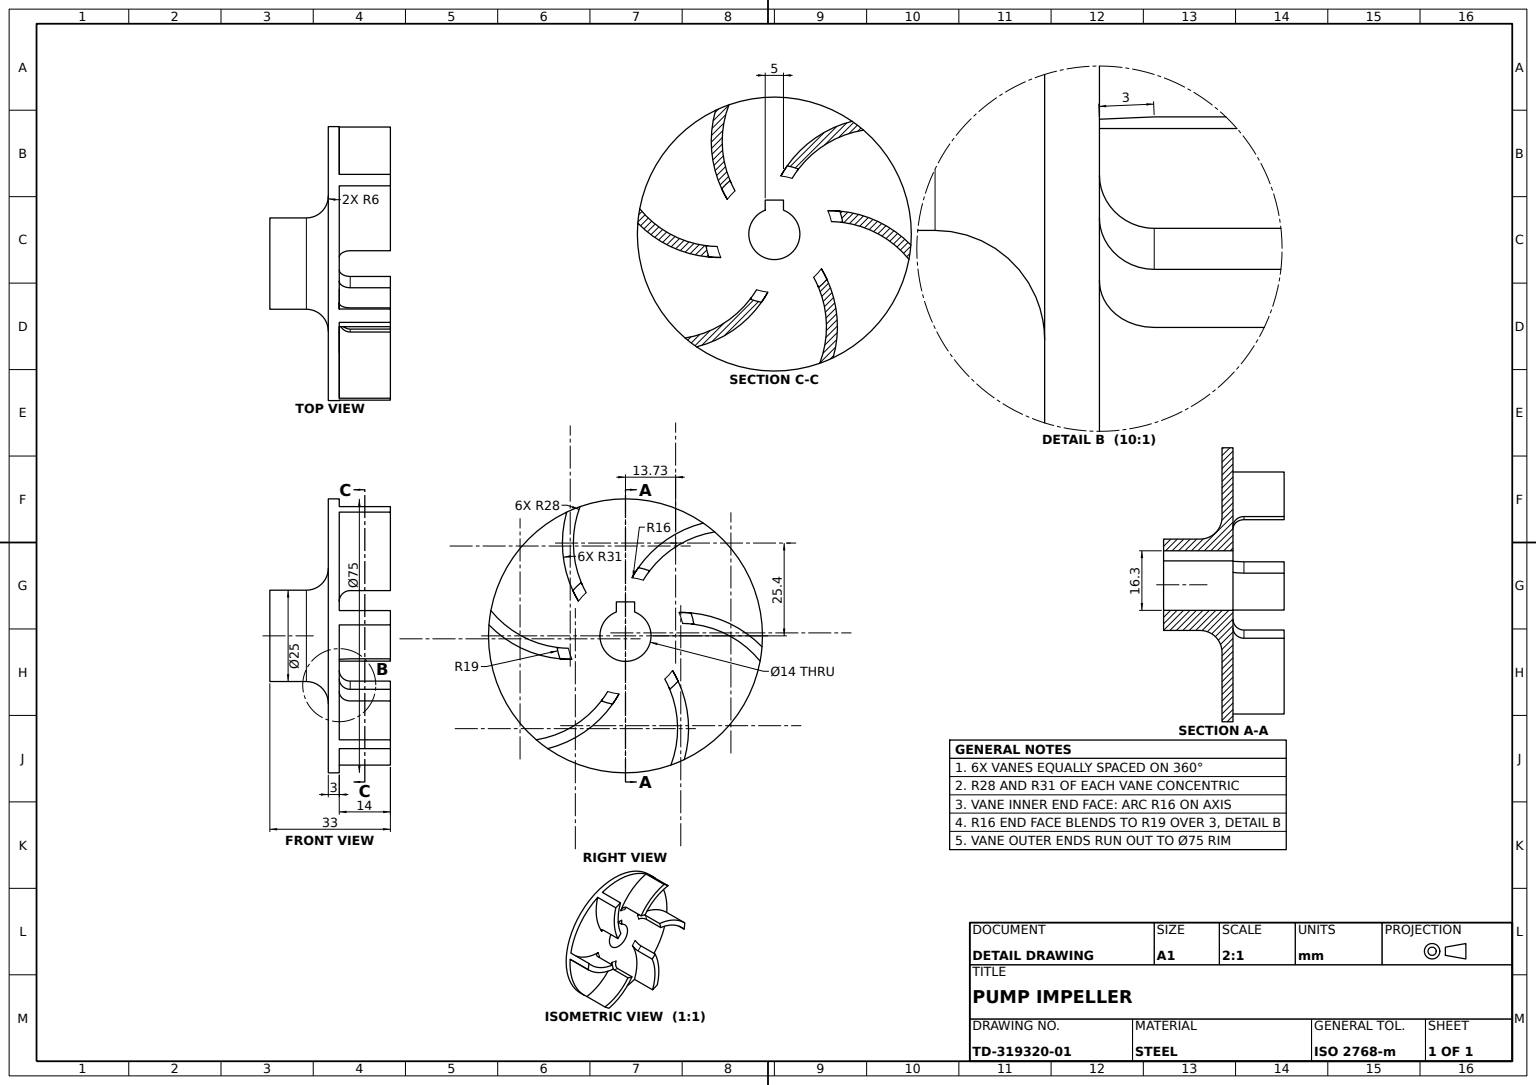
from build123d import *

# Parameters (mm, degrees)
BACK_DISC_SKETCH_R    = 37.5
BACK_DISC_75_DEPTH    = 3
HUB_SKETCH_R          = 12.5
HUB_25_DEPTH          = 16
SHAFT_START           = -16
SHAFT_BORE_DEPTH      = 16
HUB_ROOT_FILLET_R6_R  = 6
VANE_DEPTH            = 14
VANE_PATTERN_6X_COUNT = 6
VANE_FILLETS_R3_R     = 3


with BuildPart() as part:
    # Back Disc Sketch → Back Disc Ø75 (new body)
    with BuildSketch(Plane.XY):
        Circle(BACK_DISC_SKETCH_R)
        with BuildLine():
            Line((-2.5, 9.3), (2.5, 9.3))
            Line((2.5, 9.3), (2.5, 6.538348415))
            ThreePointArc((2.5, 6.538348415), (0, -7), (-2.5, 6.538348415))
            Line((-2.5, 6.538348415), (-2.5, 9.3))
        make_face(mode=Mode.SUBTRACT)
    extrude(amount=BACK_DISC_75_DEPTH)

    # Hub Sketch → Hub Ø25 (add)
    with BuildSketch(Plane(origin=(0, 0, 0), x_dir=(-1, 0, 0), z_dir=(0, 0, -1))):
        with Locations(Location((0, 0, 0), (0, 0, 180))):
            Circle(HUB_SKETCH_R)
    extrude(amount=HUB_25_DEPTH)

    # Shaft Bore Sketch → Shaft Bore (cut)
    with BuildSketch(Plane.XY.offset(SHAFT_START)):
        with BuildLine():
            Line((-2.5, 9.3), (-2.5, 6.538348415))
            ThreePointArc((-2.5, 6.538348415), (0, -7), (2.5, 6.538348415))
            Line((2.5, 6.538348415), (2.5, 9.3))
            Line((2.5, 9.3), (-2.5, 9.3))
        make_face()
    extrude(amount=SHAFT_BORE_DEPTH, mode=Mode.SUBTRACT)

    # Hub Root Fillet R6
    hub_root_fillet_r6_edges = [part.edges().sort_by_distance(p)[0] for p in [
        (-12.5, 0, 0),
    ]]
    fillet(hub_root_fillet_r6_edges, radius=HUB_ROOT_FILLET_R6_R)

    # Vane Sketch → Vane (add)
    with BuildSketch(Plane.XY.offset(3)):
        with BuildLine():
            ThreePointArc((-36.855648906, 6.92178761), (-28.764016269, 0.130807743), (-18.732180108, -3.178903649))
            ThreePointArc((-18.732180108, -3.178903649), (-18.396992291, -4.748755064), (-17.930488458, -6.284710307))
            ThreePointArc((-17.930488458, -6.284710307), (-28.487981374, -3.38694846), (-37.379807383, 3))
            ThreePointArc((-37.379807383, 3), (-37.16948812, 4.967811678), (-36.855648906, 6.92178761))
        make_face()
    vane = extrude(amount=VANE_DEPTH)

    # Vane Pattern 6x: Vane ×6 about axis
    vane_pattern_6x_axis = Axis((0, 0, 0), (0, 0, 1))
    for i in range(1, VANE_PATTERN_6X_COUNT):
        add(vane.rotate(vane_pattern_6x_axis, i * 360 / VANE_PATTERN_6X_COUNT))

    # Vane Fillets R3
    vane_fillets_r3_edges = [part.edges().sort_by_distance(p)[0] for p in [
        (-13.311038667, 13.557885145, 3),
        (-18.396992291, -4.748755064, 3),
        (-5.085953624, -18.306640209, 3),
        (13.311038667, -13.557885145, 3),
        (18.396992291, 4.748755064, 3),
        (5.085953624, 18.306640209, 3),
    ]]
    fillet(vane_fillets_r3_edges, radius=VANE_FILLETS_R3_R)


solid = part.part
